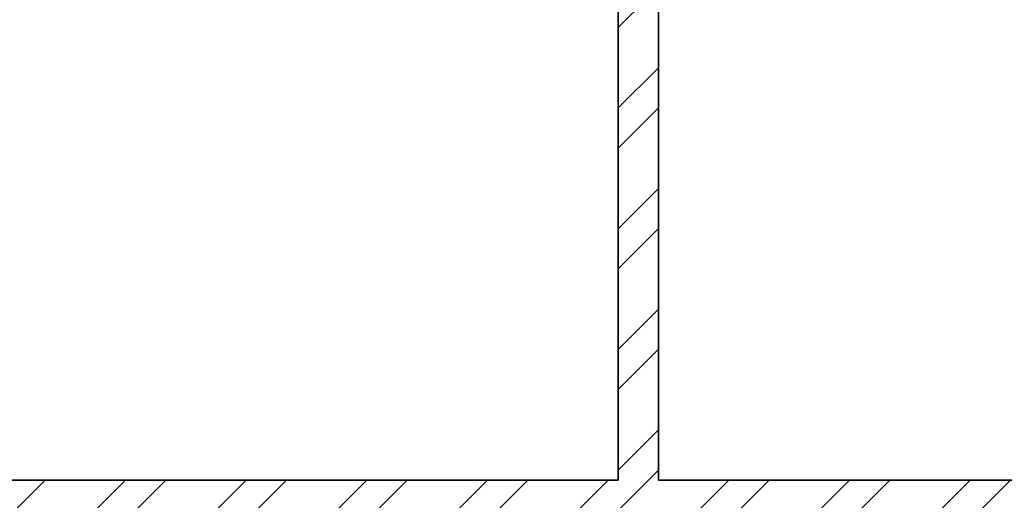
# Model space of a CAD drawing. Units: inches. Extents: x 1962 to 2771, y 1245 to 2660.
# Tile 62 of 114: x 2441 to 2551, y 1979 to 2033. Entities that reach past the tile are written whole.
import ezdxf

# ---------------------------------------------------------------- set-up
doc = ezdxf.new("R2010")
doc.units = ezdxf.units.IN
doc.layers.add('A-WALL', color=7, linetype='Continuous', lineweight=35)
doc.layers.add('A-WALL-PATT', color=252, linetype='Continuous', lineweight=13)

msp = doc.modelspace()

# ---------------------------------------------------------------- hatches: boundary and pattern name
at = {"layer": 'A-WALL-PATT'}
h = msp.add_hatch(dxfattribs=at)
h.set_pattern_fill('ANSI32', color=256)
h.paths.add_polyline_path([(2090.8074, 2467.3437), (2141.6481, 2467.3437), (2141.6481, 2469.5937), (2141.6481, 2471.8437), (2086.3074, 2471.8437), (2086.3074, 2422.5333), (2090.8074, 2422.5333)])
h.paths.add_polyline_path([(2282.7664, 2471.8437), (2204.8982, 2471.8437), (2204.8982, 2467.3437), (2234.8074, 2467.3437), (2234.8074, 2311.3437), (2228.7492, 2311.3437), (2228.7492, 2306.8437), (2234.8074, 2306.8437), (2331.9227, 2306.8437), (2331.9227, 2309.0937), (2331.9227, 2311.3437), (2239.3074, 2311.3437), (2239.3074, 2467.3437), (2282.7664, 2467.3437), (2282.7664, 2469.5937)])
h.paths.add_polyline_path([(2471.4531, 2519.8437), (2552.011, 2519.8437), (2564.3996, 2519.8437), (2564.3996, 2511.1389), (2568.8996, 2511.1389), (2568.8996, 2524.3437), (2466.9531, 2524.3437), (2466.9531, 2471.8437), (2450.0749, 2471.8437), (2446.4672, 2471.8437), (2446.4672, 2467.3437), (2450.0749, 2467.3437), (2475.9988, 2467.3437), (2475.9988, 2469.5937), (2475.9988, 2471.8437), (2471.4531, 2471.8437)])
h.paths.add_polyline_path([(2575.2231, 2469.5937), (2575.2231, 2471.8437), (2568.8996, 2471.8437), (2568.8996, 2487.1389), (2564.3996, 2487.1389), (2564.3996, 2471.8437), (2556.511, 2471.8437), (2499.2904, 2471.8437), (2499.2904, 2467.3437), (2507.8074, 2467.3437), (2507.8074, 2311.3437), (2414.863, 2311.3437), (2414.863, 2306.8437), (2512.3074, 2306.8437), (2517.0114, 2306.8437), (2517.0114, 2309.0937), (2517.0114, 2311.3437), (2512.3074, 2311.3437), (2512.3074, 2467.3437), (2575.2231, 2467.3437)])
h.paths.add_polyline_path([(2660.8074, 2471.8437), (2600.9602, 2471.8437), (2600.9602, 2467.3437), (2656.3074, 2467.3437), (2656.3074, 2432.5704), (2660.8074, 2432.5704)])
h.paths.add_polyline_path([(2660.8074, 2372.5704), (2656.3074, 2372.5704), (2656.3074, 2311.3437), (2600.276, 2311.3437), (2600.276, 2309.0937), (2600.276, 2306.8437), (2656.3074, 2306.8437), (2656.3074, 2296.2593), (2660.8074, 2296.2593)])
h.paths.add_polyline_path([(2572.3074, 2306.8437), (2577.1385, 2306.8437), (2577.1385, 2311.3437), (2551.082, 2311.3437), (2551.082, 2306.8437), (2567.8074, 2306.8437), (2567.8074, 2258.8437), (2540.0574, 2258.8437), (2540.0574, 2256.5937), (2540.0574, 2254.3437), (2567.8074, 2254.3437), (2656.3074, 2254.3437), (2656.3074, 2236.9085), (2660.8074, 2236.9085), (2660.8074, 2272.2593), (2656.3074, 2272.2593), (2656.3074, 2258.8437), (2572.3074, 2258.8437)])
h.paths.add_polyline_path([(2512.3074, 2254.3437), (2518.8716, 2254.3437), (2518.8716, 2256.5937), (2518.8716, 2258.8437), (2507.8074, 2258.8437), (2507.8074, 2177.8437), (2567.8074, 2177.8437), (2567.8074, 2172.9628), (2572.3074, 2172.9628), (2572.3074, 2177.8437), (2656.3074, 2177.8437), (2656.3074, 2166.4846), (2660.8074, 2166.4846), (2660.8074, 2200.9085), (2656.3074, 2200.9085), (2656.3074, 2182.3437), (2512.3074, 2182.3437)])
h.paths.add_polyline_path([(2656.3074, 2129.8437), (2572.3074, 2129.8437), (2572.3074, 2150.3044), (2570.0574, 2150.3044), (2567.8074, 2150.3044), (2567.8074, 2129.8437), (2507.8074, 2129.8437), (2507.8074, 2116.3027), (2510.0574, 2116.3027), (2512.3074, 2116.3027), (2512.3074, 2125.3437), (2567.8074, 2125.3437), (2572.3074, 2125.3437), (2656.3074, 2125.3437)])
h.paths.add_polyline_path([(2090.8074, 2362.5333), (2086.3074, 2362.5333), (2086.3074, 2298.6242), (2090.8074, 2298.6242), (2090.8074, 2306.8437), (2174.8074, 2306.8437), (2174.8074, 2286.4178), (2179.3074, 2286.4178), (2179.3074, 2306.8437), (2192.8641, 2306.8437), (2192.8641, 2309.0937), (2192.8641, 2311.3437), (2090.8074, 2311.3437)])
h.paths.add_polyline_path([(2209.156, 2258.8437), (2179.3074, 2258.8437), (2179.3074, 2263.2236), (2177.0574, 2263.2236), (2174.8074, 2263.2236), (2174.8074, 2258.8437), (2090.8074, 2258.8437), (2090.8074, 2274.6242), (2086.3074, 2274.6242), (2086.3074, 2238.2967), (2088.5574, 2238.2967), (2090.8074, 2238.2967), (2090.8074, 2254.3437), (2209.156, 2254.3437)])
h.paths.add_polyline_path([(2090.8074, 2177.8437), (2234.8074, 2177.8437), (2234.8074, 2173.1428), (2239.3074, 2173.1428), (2239.3074, 2258.8437), (2230.8442, 2258.8437), (2230.8442, 2256.5937), (2230.8442, 2254.3437), (2234.8074, 2254.3437), (2234.8074, 2182.3437), (2090.8074, 2182.3437), (2090.8074, 2202.2967), (2086.3074, 2202.2967), (2086.3074, 2140.0389), (2090.8074, 2140.0389)])
h.paths.add_polyline_path([(2090.8074, 2080.0389), (2086.3074, 2080.0389), (2086.3074, 2033.8437), (2090.8074, 2033.8437)], flags=17)
h.paths.add_polyline_path([(2244.9405, 2033.8437), (2239.3074, 2033.8437), (2239.3074, 2142.0665), (2237.2592, 2142.0665), (2234.8074, 2142.0665), (2234.8074, 2033.8437), (2090.8074, 2033.8437), (2076.5204, 2033.8437), (2072.0204, 2033.8437), (2072.0204, 2000.4493), (2076.5204, 2000.4493), (2076.5204, 2029.3437), (2090.8074, 2029.3437), (2244.9405, 2029.3437), (2244.9405, 2031.5937)])
h.paths.add_polyline_path([(2234.8074, 1933.3437), (2076.5204, 1933.3437), (2076.5204, 1952.4493), (2074.2704, 1952.4493), (2072.0204, 1952.4493), (2072.0204, 1933.3437), (2072.0204, 1928.8437), (2234.8074, 1928.8437)])
h.paths.add_polyline_path([(2090.8074, 1928.8437), (2086.3074, 1928.8437), (2086.3074, 1906.5013), (2090.8074, 1906.5013)])
h.paths.add_polyline_path([(2090.8074, 1846.5013), (2086.3074, 1846.5013), (2086.3074, 1769.9917), (2088.5574, 1769.9917), (2090.8074, 1769.9917), (2090.8074, 1780.3437), (2234.8074, 1780.3437), (2234.8074, 1708.3437), (2230.3764, 1708.3437), (2230.3764, 1703.8437), (2239.3074, 1703.8437), (2239.3074, 1792.6669), (2237.0574, 1792.6669), (2234.8074, 1792.6669), (2234.8074, 1784.8437), (2090.8074, 1784.8437)])
h.paths.add_polyline_path([(2239.3074, 1928.8437), (2244.9405, 1928.8437), (2244.9405, 1931.0937), (2244.9405, 1933.3437), (2234.8074, 1933.3437), (2234.8074, 1928.8437), (2234.8074, 1825.5949), (2239.3074, 1825.5949)])
h.paths.add_polyline_path([(2148.0425, 1649.0937), (2148.0425, 1651.3437), (2090.8074, 1651.3437), (2090.8074, 1646.8437), (2148.0425, 1646.8437)], flags=0)
h.paths.add_polyline_path([(2207.5601, 1708.3437), (2090.8074, 1708.3437), (2090.8074, 1703.8437), (2174.8074, 1703.8437), (2174.8074, 1651.3437), (2170.4457, 1651.3437), (2170.4457, 1646.8437), (2195.9924, 1646.8437), (2195.9924, 1649.0937), (2195.9924, 1651.3437), (2179.3074, 1651.3437), (2179.3074, 1703.8437), (2207.5601, 1703.8437), (2207.5601, 1706.0937)])
h.paths.add_polyline_path([(2090.8074, 1733.9917), (2086.3074, 1733.9917), (2086.3074, 1696.1032), (2088.5574, 1696.1032), (2090.8074, 1696.1032)])
h.paths.add_polyline_path([(2090.8074, 1672.1032), (2086.3074, 1672.1032), (2086.3074, 1600.3335), (2090.8074, 1600.3335)])
h.paths.add_polyline_path([(2090.8074, 1540.3335), (2086.3074, 1540.3335), (2086.3074, 1486.3437), (2139.6766, 1486.3437), (2139.6766, 1490.8437), (2090.8074, 1490.8437)])
h.paths.add_polyline_path([(2302.3876, 1490.8437), (2239.3074, 1490.8437), (2239.3074, 1646.8437), (2335.9994, 1646.8437), (2335.9994, 1651.3437), (2229.884, 1651.3437), (2229.884, 1646.8437), (2234.8074, 1646.8437), (2234.8074, 1490.8437), (2202.7103, 1490.8437), (2202.7103, 1488.5937), (2202.7103, 1486.3437), (2275.0699, 1486.3437), (2275.0699, 1475.772), (2279.5699, 1475.772), (2279.5699, 1486.3437), (2302.3876, 1486.3437)])
h.paths.add_polyline_path([(2279.5699, 1451.772), (2275.0699, 1451.772), (2275.0699, 1438.3437), (2174.8074, 1438.3437), (2174.8074, 1486.3437), (2179.7922, 1486.3437), (2179.7922, 1490.8437), (2163.3585, 1490.8437), (2163.3585, 1488.5937), (2163.3585, 1486.3437), (2170.3074, 1486.3437), (2170.3074, 1433.8437), (2279.5699, 1433.8437)])
h.paths.add_polyline_path([(2427.2363, 1490.8437), (2375.8074, 1490.8437), (2375.8074, 1646.8437), (2381.6401, 1646.8437), (2381.6401, 1651.3437), (2365.887, 1651.3437), (2365.887, 1649.0937), (2365.887, 1646.8437), (2371.3074, 1646.8437), (2371.3074, 1490.8437), (2327.5627, 1490.8437), (2327.5627, 1488.5937), (2327.5627, 1486.3437), (2371.3074, 1486.3437), (2371.3074, 1433.8437), (2375.8074, 1433.8437), (2375.8074, 1486.3437), (2427.2363, 1486.3437)])
h.paths.add_polyline_path([(2512.3074, 1646.8437), (2519.4351, 1646.8437), (2519.4351, 1649.0937), (2519.4351, 1651.3437), (2507.8074, 1651.3437), (2416.0063, 1651.3437), (2416.0063, 1649.0937), (2416.0063, 1646.8437), (2507.8074, 1646.8437), (2507.8074, 1490.8437), (2497.0532, 1490.8437), (2497.0532, 1488.5937), (2497.0532, 1486.3437), (2574.9344, 1486.3437), (2574.9344, 1476.0181), (2579.4344, 1476.0181), (2579.4344, 1486.3437), (2584.4872, 1486.3437), (2584.3074, 1490.8437), (2512.3074, 1490.8437)])
h.paths.add_polyline_path([(2470.5091, 1486.3437), (2473.9767, 1486.3437), (2473.9767, 1490.8437), (2449.6605, 1490.8437), (2449.6605, 1488.5937), (2449.6605, 1486.3437), (2466.0091, 1486.3437), (2466.0091, 1433.8437), (2470.5091, 1433.8437), (2579.4344, 1433.8437), (2579.4344, 1452.0181), (2574.9344, 1452.0181), (2574.9344, 1438.3437), (2554.5091, 1438.3437), (2470.5091, 1438.3437)])
h.paths.add_polyline_path([(2656.3074, 1490.8437), (2611.86, 1490.8437), (2611.86, 1486.3437), (2656.3074, 1486.3437)])
h.paths.add_polyline_path([(2660.8074, 1532.7007), (2658.5574, 1532.7007), (2656.3074, 1532.7007), (2656.3074, 1486.3437), (2660.8074, 1486.3437)])
h.paths.add_polyline_path([(2660.8074, 1664.9663), (2656.3074, 1664.9663), (2656.3074, 1651.3437), (2602.2313, 1651.3437), (2602.2313, 1646.8437), (2656.3074, 1646.8437), (2656.3074, 1592.7007), (2660.8074, 1592.7007)])
h.paths.add_polyline_path([(2660.8074, 1724.5221), (2656.3074, 1724.5221), (2656.3074, 1703.8437), (2542.4725, 1703.8437), (2542.4725, 1699.3437), (2567.8074, 1699.3437), (2567.8074, 1651.3437), (2552.7766, 1651.3437), (2552.7766, 1649.0937), (2552.7766, 1646.8437), (2577.2878, 1646.8437), (2577.2878, 1649.0937), (2577.2878, 1651.3437), (2572.3074, 1651.3437), (2572.3074, 1699.3437), (2656.3074, 1699.3437), (2656.3074, 1688.9663), (2660.8074, 1688.9663)])
h.paths.add_polyline_path([(2660.8074, 1880.6524), (2656.3074, 1880.6524), (2656.3074, 1832.8437), (2512.3074, 1832.8437), (2512.3074, 1837.8959), (2507.8074, 1837.8959), (2507.8074, 1828.3437), (2567.8074, 1828.3437), (2567.8074, 1804.3437), (2572.3074, 1804.3437), (2572.3074, 1828.3437), (2656.3074, 1828.3437), (2656.3074, 1818.6778), (2660.8074, 1818.6778)])
h.paths.add_polyline_path([(2660.8074, 1794.6778), (2656.3074, 1794.6778), (2656.3074, 1780.3437), (2572.3074, 1780.3437), (2572.3074, 1783.0303), (2570.0574, 1783.0303), (2567.8074, 1783.0303), (2567.8074, 1780.3437), (2507.8074, 1780.3437), (2507.8074, 1699.3437), (2517.8858, 1699.3437), (2517.8858, 1701.5937), (2517.8858, 1703.8437), (2512.3074, 1703.8437), (2512.3074, 1775.8437), (2656.3074, 1775.8437), (2656.3074, 1760.5221), (2660.8074, 1760.5221)])
h.paths.add_polyline_path([(2660.8074, 1981.3437), (2660.8074, 2020.2808), (2658.5574, 2020.2808), (2656.3074, 2020.2808), (2656.3074, 1981.3437), (2512.3074, 1981.3437), (2512.3074, 2086.6996), (2507.8074, 2086.6996), (2507.8074, 1981.3437), (2375.8074, 1981.3437), (2375.8074, 1986.8505), (2373.5574, 1986.8505), (2371.3074, 1986.8505), (2371.3074, 1973.2607), (2375.8074, 1973.2607), (2375.8074, 1976.8437), (2507.8074, 1976.8437), (2507.8074, 1865.4281), (2510.0574, 1865.4281), (2512.3074, 1865.4281), (2512.3074, 1976.8437), (2660.8074, 1976.8437)])
h.paths.add_polyline_path([(2375.8074, 1940.297), (2373.5574, 1940.297), (2371.3074, 1940.297), (2371.3074, 1933.3437), (2278.4434, 1933.3437), (2278.4434, 1928.8437), (2371.3074, 1928.8437), (2371.3074, 1651.3437), (2375.8074, 1651.3437)])
h.paths.add_polyline_path([(2660.8074, 1976.8437), (2656.3074, 1976.8437), (2656.3074, 1940.6524), (2660.8074, 1940.6524)], flags=17)
h.paths.add_polyline_path([(2660.8074, 2142.4846), (2656.3074, 2142.4846), (2656.3074, 2080.2808), (2660.8074, 2080.2808)])
h.paths.add_polyline_path([(2381.4189, 2311.3437), (2375.8074, 2311.3437), (2375.8074, 2467.3437), (2424.7242, 2467.3437), (2424.7242, 2469.5937), (2424.7242, 2471.8437), (2375.8074, 2471.8437), (2375.8074, 2524.3437), (2371.3074, 2524.3437), (2371.3074, 2471.8437), (2307.2097, 2471.8437), (2307.2097, 2467.3437), (2371.3074, 2467.3437), (2371.3074, 2311.3437), (2366.8901, 2311.3437), (2366.8901, 2306.8437), (2371.3074, 2306.8437), (2371.3074, 2033.8437), (2279.6589, 2033.8437), (2279.6589, 2029.3437), (2371.3074, 2029.3437), (2371.3074, 2014.2598), (2375.8074, 2014.2598), (2375.8074, 2306.8437), (2381.4189, 2306.8437)])
h.paths.add_polyline_path([(2263.3074, 2524.3437), (2170.3074, 2524.3437), (2170.3074, 2519.8437), (2170.3074, 2471.8437), (2165.0312, 2471.8437), (2165.0312, 2467.3437), (2179.6721, 2467.3437), (2179.6721, 2469.5161), (2179.6721, 2471.8437), (2174.8074, 2471.8437), (2174.8074, 2519.8437), (2258.8074, 2519.8437), (2258.8074, 2511.6436), (2263.3074, 2511.6436)])
h.paths.add_polyline_path([(2245.0232, 1361.4123), (2492.9468, 1361.4123), (2492.9468, 1398.505), (2245.0232, 1398.505)], flags=9)
h.paths.add_polyline_path([(2388.1434, 2086.6936), (2425.0704, 2086.6936), (2425.0704, 2105.3509), (2388.1434, 2105.3509)], flags=9)
h.paths.add_polyline_path([(2404.922, 2242.6744), (2445.7337, 2242.6744), (2445.7337, 2261.3318), (2404.922, 2261.3318)], flags=9)
h.paths.add_polyline_path([(2269.4107, 2156.7935), (2306.3378, 2156.7935), (2306.3378, 2175.4508), (2269.4107, 2175.4508)], flags=9)
h.paths.add_polyline_path([(2269.3277, 2233.4343), (2306.2547, 2233.4343), (2306.2547, 2252.0917), (2269.3277, 2252.0917)], flags=9)
h.paths.add_polyline_path([(2431.6052, 2320.6922), (2470.4456, 2320.6922), (2470.4456, 2339.3495), (2431.6052, 2339.3495)], flags=25)
h.paths.add_polyline_path([(2249.6902, 2315.7608), (2288.5306, 2315.7608), (2288.5306, 2334.4182), (2249.6902, 2334.4182)], flags=25)
h.paths.add_polyline_path([(2096.9301, 2314.3181), (2135.7704, 2314.3181), (2135.7704, 2332.9755), (2096.9301, 2332.9755)], flags=25)
h.paths.add_polyline_path([(2134.3475, 2285.7089), (2161.4655, 2285.7089), (2161.4655, 2304.3662), (2134.3475, 2304.3662)], flags=9)
h.paths.add_polyline_path([(2126.5155, 2209.4076), (2159.9227, 2209.4076), (2159.9227, 2228.065), (2126.5155, 2228.065)], flags=25)
h.paths.add_polyline_path([(2110.5753, 2141.5299), (2149.4157, 2141.5299), (2149.4157, 2160.1872), (2110.5753, 2160.1872)], flags=25)
h.paths.add_polyline_path([(2249.8618, 1968.3317), (2286.3966, 1968.3317), (2286.3966, 1986.989), (2249.8618, 1986.989)], flags=9)
h.paths.add_polyline_path([(2395.9507, 1777.0051), (2436.7624, 1777.0051), (2436.7624, 1795.6625), (2395.9507, 1795.6625)], flags=9)
h.paths.add_polyline_path([(2398.5259, 1888.5651), (2435.0062, 1888.5651), (2435.0062, 1907.2224), (2398.5259, 1907.2224)], flags=25)
h.paths.add_polyline_path([(2259.3506, 1728.3559), (2296.2776, 1728.3559), (2296.2776, 1747.0132), (2259.3506, 1747.0132)], flags=9)
h.paths.add_polyline_path([(2271.3698, 1845.268), (2308.2968, 1845.268), (2308.2968, 1863.9253), (2271.3698, 1863.9253)], flags=9)
h.paths.add_polyline_path([(2120.9355, 1786.3027), (2159.7759, 1786.3027), (2159.7759, 1804.9601), (2120.9355, 1804.9601)], flags=25)
h.paths.add_polyline_path([(2121.3164, 1732.1043), (2154.7236, 1732.1043), (2154.7236, 1750.7616), (2121.3164, 1750.7616)], flags=25)
h.paths.add_polyline_path([(2118.3706, 1678.8997), (2147.5282, 1678.8997), (2147.5282, 1697.557), (2118.3706, 1697.557)], flags=25)
h.paths.add_polyline_path([(2385.9227, 1493.557), (2424.763, 1493.557), (2424.763, 1512.2143), (2385.9227, 1512.2143)], flags=25)
h.paths.add_polyline_path([(2248.7058, 1500.0256), (2287.5462, 1500.0256), (2287.5462, 1518.6829), (2248.7058, 1518.6829)], flags=25)
h.paths.add_polyline_path([(2104.1669, 1617.3771), (2143.0073, 1617.3771), (2143.0073, 1636.0344), (2104.1669, 1636.0344)], flags=9)
h.paths.add_polyline_path([(2096.0714, 1447.8824), (2137.3845, 1447.8824), (2137.3845, 1458.1859), (2096.0714, 1458.1859)], flags=9)
h.paths.add_polyline_path([(2180.6114, 1440.325), (2209.7689, 1440.325), (2209.7689, 1458.9823), (2180.6114, 1458.9823)], flags=25)
h.paths.add_polyline_path([(2316.1698, 1447.9637), (2357.4829, 1447.9637), (2357.4829, 1458.2673), (2316.1698, 1458.2673)], flags=9)
h.paths.add_polyline_path([(2397.6187, 1447.9637), (2438.9318, 1447.9637), (2438.9318, 1458.2673), (2397.6187, 1458.2673)], flags=9)
h.paths.add_polyline_path([(2473.0778, 1439.5953), (2502.2354, 1439.5953), (2502.2354, 1458.2527), (2473.0778, 1458.2527)], flags=25)
h.paths.add_polyline_path([(2589.7027, 1447.8819), (2631.0158, 1447.8819), (2631.0158, 1458.1855), (2589.7027, 1458.1855)], flags=9)
h.paths.add_polyline_path([(2522.4009, 1497.5285), (2561.2413, 1497.5285), (2561.2413, 1516.1859), (2522.4009, 1516.1859)], flags=25)
h.paths.add_polyline_path([(2579.6565, 1671.3482), (2608.8141, 1671.3482), (2608.8141, 1690.0056), (2579.6565, 1690.0056)], flags=25)
h.paths.add_polyline_path([(2544.7038, 1725.5064), (2578.1111, 1725.5064), (2578.1111, 1744.1637), (2544.7038, 1744.1637)], flags=25)
h.paths.add_polyline_path([(2578.1191, 1807.472), (2607.2766, 1807.472), (2607.2766, 1826.1293), (2578.1191, 1826.1293)], flags=25)
h.paths.add_polyline_path([(2595.0614, 1835.1839), (2633.9018, 1835.1839), (2633.9018, 1853.8413), (2595.0614, 1853.8413)], flags=25)
h.paths.add_polyline_path([(2567.0097, 2097.7035), (2605.8501, 2097.7035), (2605.8501, 2116.3609), (2567.0097, 2116.3609)], flags=9)
h.paths.add_polyline_path([(2586.644, 2134.6454), (2615.8015, 2134.6454), (2615.8015, 2153.3027), (2586.644, 2153.3027)], flags=9)
h.paths.add_polyline_path([(2544.6185, 2212.6783), (2578.0258, 2212.6783), (2578.0258, 2231.3356), (2544.6185, 2231.3356)], flags=25)
h.paths.add_polyline_path([(2577.0273, 2256.9023), (2606.1849, 2256.9023), (2606.1849, 2275.5597), (2577.0273, 2275.5597)], flags=24)
h.paths.add_polyline_path([(2605.2683, 2315.2821), (2644.1087, 2315.2821), (2644.1087, 2333.9395), (2605.2683, 2333.9395)], flags=25)
h.paths.add_polyline_path([(2583.1244, 2496.1815), (2624.4375, 2496.1815), (2624.4375, 2506.4851), (2583.1244, 2506.4851)], flags=9)
h.paths.add_polyline_path([(2474.761, 2497.0823), (2503.9185, 2497.0823), (2503.9185, 2515.7397), (2474.761, 2515.7397)], flags=25)
h.paths.add_polyline_path([(2387.5787, 2494.2563), (2428.902, 2494.2563), (2428.902, 2504.5598), (2387.5787, 2504.5598)], flags=9)
h.paths.add_polyline_path([(2300.1657, 2500.1564), (2341.4788, 2500.1564), (2341.4788, 2510.46), (2300.1657, 2510.46)], flags=25)
h.paths.add_polyline_path([(2176.8589, 2497.5843), (2206.0165, 2497.5843), (2206.0165, 2516.2416), (2176.8589, 2516.2416)], flags=25)
h.paths.add_polyline_path([(2097.4668, 2494.9762), (2138.7799, 2494.9762), (2138.7799, 2505.2798), (2097.4668, 2505.2798)], flags=9)

# ---------------------------------------------------------------- linework, layer by layer
at = {"layer": 'A-WALL'}
for p, q in [((2512.3074, 2088.0256), (2512.3074, 1981.3437)), ((2507.8074, 2086.6996), (2507.8074, 1981.3437)), ((2507.8074, 2086.6996), (2507.8074, 1981.3437)), ((2375.8074, 1981.3437), (2507.8074, 1981.3437)), ((2512.3074, 1981.3437), (2656.3074, 1981.3437))]:
    msp.add_line(p, q, dxfattribs=at)

doc.saveas('drawing.dxf')
